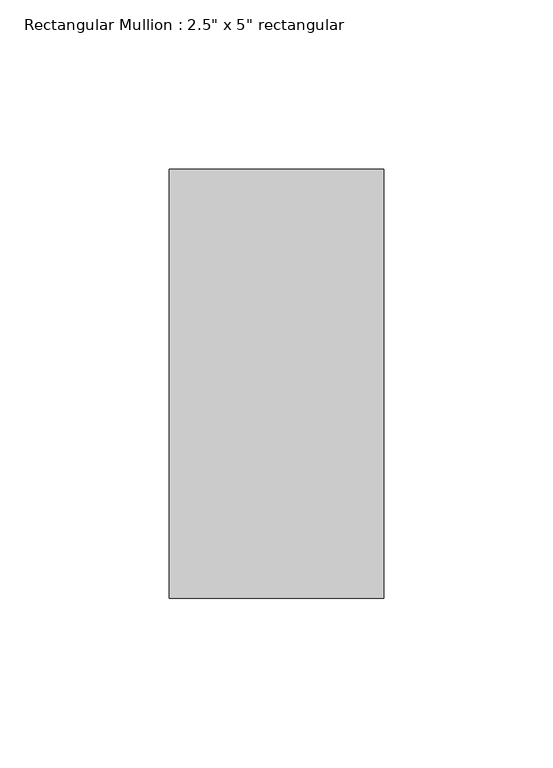
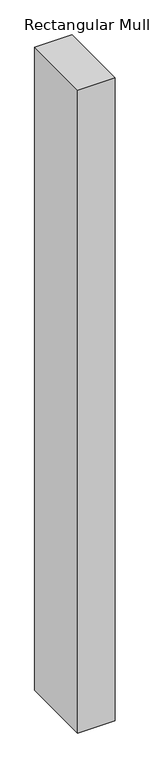
"""IFC4 building model written with IfcOpenShell, lengths in millimetres: member geometry."""

from ifc_helpers import new_model, si_unit, frame, origin, place, context, project, spatial, polyline, outline, extrude, source, transform, mapped, element, save


def member_f4ce465c(model_context):
    return source(origin(), model_context, "Body", "SweptSolid", [
        extrude(outline(polyline([(31.75, 63.5), (31.75, -63.5), (-31.75, -63.5), (-31.75, 63.5), (31.75, 63.5)])), frame((0.0, 0.0, -1157.2424454), z_axis=(0.0, 0.0, 1.0), x_axis=(1.0, 0.0, 0.0)), (0.0, 0.0, 1.0), 1157.2424454),
    ])


if __name__ == "__main__":
    model = new_model("IFC4")
    model_context = context("Model", 3, world=origin())
    ifc_project = project(units=[si_unit("LENGTHUNIT", "METRE", prefix="MILLI")], contexts=[model_context])
    site = spatial("IfcSite", under=ifc_project)
    building = spatial("IfcBuilding", under=site)
    placement = place(None, origin())
    member_shape = member_f4ce465c(model_context)
    element("IfcMember", 1, ObjectType="Rectangular Mullion : 2.5\" x 5\" rectangular", at=placement, inside=building, context=model_context, shape_type="MappedRepresentation", body=[
        mapped(member_shape, transform((0.0, 0.0, 0.0), x_axis=(1.0, 0.0, 0.0), y_axis=(0.0, 1.0, 0.0), z_axis=(0.0, 0.0, 1.0))),
    ])
    save(model, "model.ifc")

# Revit data of these elements
# Type "Rectangular Mullion : 2.5\" x 5\" rectangular"
#   built-in parameter 1007304 = 0.416667 (stored number, unit not read)
#   built-in parameter 1007301 = 0.104167 (stored number, unit not read)
#   built-in parameter 1007300 = 0.104167 (stored number, unit not read)
# Element 1 (IfcMember, "Rectangular Mullion : 2.5\" x 5\" rectangular")
#   Materials on its faces: "BLACK COLOUR"
# Materials
#   "BLACK COLOUR": class "Generic", colour RGB 120 120 120, transparency 0, Cost = 0
